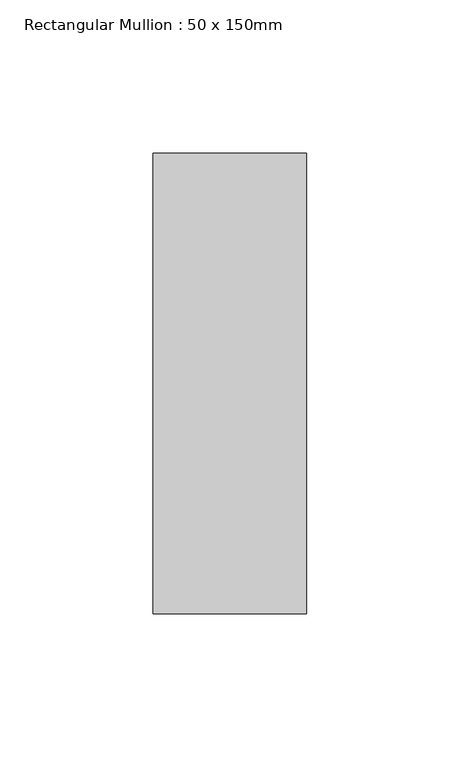
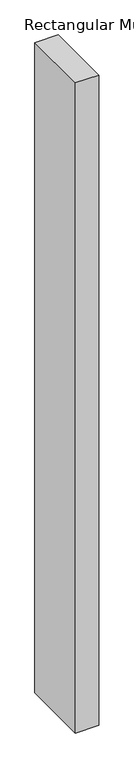
"""IFC4 building model written with IfcOpenShell, lengths in millimetres: member geometry, Rectangular Mullion : 50 x 150mm."""

from ifc_helpers import new_model, si_unit, frame, origin, place, context, project, spatial, polyline, outline, extrude, source, transform, mapped, element, save


def rectangular_mullion_50_x_150mm_4a18de0c(model_context):
    return source(origin(), model_context, "Body", "SweptSolid", [
        extrude(outline(polyline([(0.0, 75.0), (0.0, -75.0), (-50.0, -75.0), (-50.0, 75.0), (0.0, 75.0)])), frame((0.0, 0.0, -1466.6666665), z_axis=(0.0, 0.0, 1.0), x_axis=(1.0, 0.0, 0.0)), (0.0, 0.0, 1.0), 1466.6666665),
    ])


if __name__ == "__main__":
    model = new_model("IFC4")
    model_context = context("Model", 3, world=origin())
    ifc_project = project(units=[si_unit("LENGTHUNIT", "METRE", prefix="MILLI")], contexts=[model_context])
    site = spatial("IfcSite", under=ifc_project)
    building = spatial("IfcBuilding", under=site)
    placement = place(None, origin())
    rectangular_mullion_50_x_150mm_shape = rectangular_mullion_50_x_150mm_4a18de0c(model_context)
    element("IfcMember", 1, ObjectType="Rectangular Mullion : 50 x 150mm", at=placement, inside=building, context=model_context, shape_type="MappedRepresentation", body=[
        mapped(rectangular_mullion_50_x_150mm_shape, transform((0.0, 0.0, 0.0), x_axis=(1.0, 0.0, 0.0), y_axis=(0.0, 1.0, 0.0), z_axis=(0.0, 0.0, 1.0))),
    ])
    save(model, "model.ifc")

# Revit data of these elements
# Type "Rectangular Mullion : 50 x 150mm"
#   built-in parameter 1007304 = 0.492126 (stored number, unit not read)
#   built-in parameter 1007301 = 0.082021 (stored number, unit not read)
#   built-in parameter 1007300 = 0.082021 (stored number, unit not read)
# Element 1 (IfcMember, "Rectangular Mullion : 50 x 150mm")
#   Materials on its faces: "Aluminium"
# Materials
#   "Aluminium": class "Metal", colour RGB 247 247 247, transparency 0, Description = "Aluminium 6061", Cost = 0
